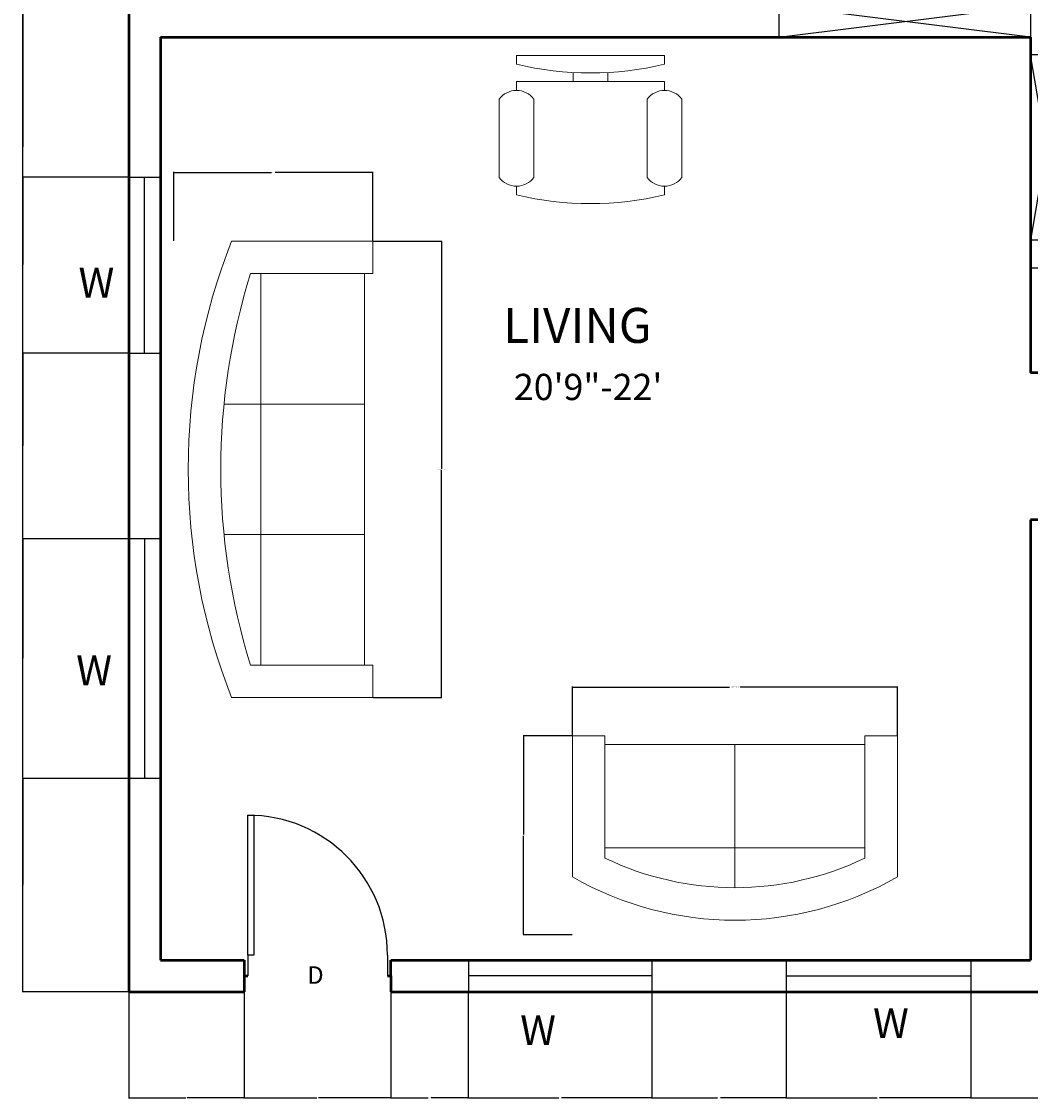
# Model space of a CAD drawing. Units: inches. Extents: x 2164 to 3752, y 2015 to 2629.
# Tile 5 of 8: x 3295 to 3583, y 2015 to 2323. Entities that reach past the tile are written whole.
import ezdxf
from ezdxf.enums import TextEntityAlignment as Align

# ---------------------------------------------------------------- set-up
doc = ezdxf.new("R2010")
doc.units = ezdxf.units.IN
for name, color, linetype, lineweight in [('A-ANNO-DIMS', 2, 'Continuous', 18), ('A-ANNO-TEXT', 7, 'Continuous', 25), ('A-AREA-IDEN', 3, 'Continuous', 25), ('A-DOOR', 3, 'Continuous', 25), ('A-FURN', 8, 'Continuous', 18), ('A-GLAZ', 4, 'Continuous', 25), ('A-WALL', 7, 'Continuous', 50)]:
    doc.layers.add(name, color=color, linetype=linetype, lineweight=lineweight)
doc.styles.get("Standard").update_dxf_attribs({"font": 'arial.ttf'})
doc.dimstyles.get("Standard").update_dxf_attribs({"dimtxt": 0.18, "dimasz": 0.18, "dimexe": 0.18, "dimexo": 0.0625, "dimgap": 0.09, "dimtad": 0, "dimtih": 1, "dimtoh": 1, "dimdec": 4, "dimzin": 0, "dimdsep": 46, "dimtxsty": 'Standard', "dimcen": 0.09, "dimadec": 0, "dimazin": 0, "dimtfac": 1, "dimtdec": 4, "dimtofl": 0, "dimtmove": 0, "dimatfit": 3, "dimfxl": 1, "dimtolj": 1, "dimtzin": 0, "dimarcsym": 0})

# ---------------------------------------------------------------- blocks, each defined once
blk = doc.blocks.new('*U7')
for p, q in [((0, 0), (0, -6)), ((40, 0), (40, -6))]:
    blk.add_line(p, q)
blk.add_lwpolyline([(0, 0), (0, 40), (1.75, 40), (1.75, 0)], close=True)
blk.add_arc((0, 0), 40, 0, 90)
blk = doc.blocks.new('Sofa - Roundback 7 ft.')
for p, q in [((-12.00002, -32.4421), (-12.00003, -6.5971)), ((11.99997, -32.4421), (11.99998, -6.5971)), ((-36.000027, -34), (-36.000027, -11.4696)), ((35.99998, -34), (35.99998, -11.4696)), ((-35.999844, -13.3819), (35.9998, -13.3819)), ((-36.000027, -32.4421), (35.99998, -32.4421))]:
    blk.add_line(p, q)
for points in [[(-36.000027, -34), (-42.000027, -34), (-42.000027, -8)], [(41.99998, -8), (41.99998, -34), (35.99998, -34)]]:
    blk.add_lwpolyline(points)
for centre, radius, start, end in [((0, -114.25), 114.25, 68.43141, 111.5686), ((-0.00001, -127.1968), 121.1968, 72.72033, 107.2797)]:
    blk.add_arc(centre, radius, start, end)
blk = doc.blocks.new('Sofa - Roundback Loveseat 5 ft.')
for p, q in [((0, -32.44198), (0, -5.99998)), ((-24, -33.99998), (-24, -11.46958)), ((24.00004, -33.99998), (24.00004, -11.46958)), ((-23.9998, -13.38178), (23.99986, -13.38178)), ((-24, -32.44198), (24.00004, -32.44198))]:
    blk.add_line(p, q)
for points in [[(-24, -33.99998), (-30, -33.99998), (-30, -7.99998)], [(30.00004, -7.99998), (30.00004, -33.99998), (24.00004, -33.99998)]]:
    blk.add_lwpolyline(points)
for centre, radius, start, end in [((0, -60.24998), 60.24998, 60.13715, 119.8628), ((0, -61.38438), 55.38444, 64.32083, 115.6792)]:
    blk.add_arc(centre, radius, start, end)
blk = doc.blocks.new('Chair - Desk')
for p, q in [((-8.5, 0), (-8.5, -1)), ((-8.5, 0), (8.5, 0)), ((8.5, 0), (8.5, -1)), ((-2, -3), (-2, -1.9355)), ((2, -1.9576), (2, -3)), ((-8.5, -3), (-8.5, -4)), ((-8.5, -3), (8.5, -3)), ((8.5, -3), (8.5, -4)), ((-10.5, -5), (-10.5, -14)), ((-6.5, -14), (-6.5, -5)), ((6.5, -5), (6.5, -14)), ((10.5, -14), (10.5, -5)), ((-8.5, -15), (-8.5, -16)), ((8.5, -15), (8.5, -16))]:
    blk.add_line(p, q)
for centre, radius, start, end in [((0, 34.625), 36.625, 256.5803, 283.4197), ((-8.5, -6.5), 2.5, 36.8699, 143.1301), ((8.5, -6.5), 2.5, 36.8699, 143.1301), ((-8.5, -12.5), 2.5, 216.8699, 323.1301), ((8.5, -12.5), 2.5, 216.8699, 323.1301), ((0, 19.625), 36.625, 256.5803, 283.4197)]:
    blk.add_arc(centre, radius, start, end)
blk = doc.blocks.new('VENT-OPENING')
for p, q in [((9, 53), (0, 53)), ((9, 53), (0, 0)), ((9, 0), (0, 53)), ((9, 0), (0, 0))]:
    blk.add_line(p, q)
blk = doc.blocks.new('*D27')
at = {"layer": 'A-ANNO-DIMS', "color": 0, "lineweight": -2, "transparency": 16777216}
for p, q in [((3395.28, 2260.44), (3414.99, 2260.44)), ((3414.81, 2260.26), (3414.81, 2195.32)), ((3414.81, 2130.01), (3414.81, 2194.95)), ((3395.28, 2129.83), (3414.99, 2129.83))]:
    blk.add_line(p, q, dxfattribs=at)
at = {"layer": 'A-ANNO-DIMS', "color": 0, "transparency": 16777216}
for points in [[(3414.78, 2260.26), (3414.84, 2260.26), (3414.81, 2260.44)], [(3414.78, 2130.01), (3414.84, 2130.01), (3414.81, 2129.83)]]:
    blk.add_solid(points, dxfattribs=at)
at = {"layer": 'Defpoints', "color": 0, "transparency": 16777216}
for p in [(3395.22, 2260.44), (3414.81, 2260.44), (3395.22, 2129.83)]:
    blk.add_point(p, dxfattribs=at)
at = {"layer": 'A-ANNO-DIMS', "color": 0, "transparency": 16777216, "insert": (3414.81, 2195.13), "char_height": 0.18, "attachment_point": 5}
blk.add_mtext('\\A1;SOFA 7 FT 131 TYP.', dxfattribs=at)
blk = doc.blocks.new('*D28')
at = {"layer": 'A-ANNO-DIMS', "color": 0, "lineweight": -2, "transparency": 16777216}
for p, q in [((3338.21, 2260.5), (3338.21, 2280.21)), ((3338.39, 2280.03), (3366.19, 2280.03)), ((3395.04, 2280.03), (3367.24, 2280.03)), ((3395.22, 2260.5), (3395.22, 2280.21))]:
    blk.add_line(p, q, dxfattribs=at)
at = {"layer": 'A-ANNO-DIMS', "color": 0, "transparency": 16777216}
for points in [[(3338.39, 2280.06), (3338.39, 2280), (3338.21, 2280.03)], [(3395.04, 2280.06), (3395.04, 2280), (3395.22, 2280.03)]]:
    blk.add_solid(points, dxfattribs=at)
at = {"layer": 'Defpoints', "color": 0, "transparency": 16777216}
for p in [(3338.21, 2280.03), (3338.21, 2260.44), (3395.22, 2260.44)]:
    blk.add_point(p, dxfattribs=at)
at = {"layer": 'A-ANNO-DIMS', "color": 0, "transparency": 16777216, "insert": (3366.72, 2280.03), "char_height": 0.18, "attachment_point": 5}
blk.add_mtext('\\A1;57 TYP.', dxfattribs=at)
blk = doc.blocks.new('*D29')
at = {"layer": 'A-ANNO-DIMS', "color": 0, "lineweight": -2, "transparency": 16777216}
for p, q in [((3452.32, 2118.94), (3452.32, 2133.02)), ((3452.5, 2132.84), (3497.31, 2132.84)), ((3545.16, 2132.84), (3500.34, 2132.84)), ((3545.34, 2118.94), (3545.34, 2133.02))]:
    blk.add_line(p, q, dxfattribs=at)
at = {"layer": 'A-ANNO-DIMS', "color": 0, "transparency": 16777216}
for points in [[(3452.5, 2132.87), (3452.5, 2132.81), (3452.32, 2132.84)], [(3545.16, 2132.87), (3545.16, 2132.81), (3545.34, 2132.84)]]:
    blk.add_solid(points, dxfattribs=at)
at = {"layer": 'Defpoints', "color": 0, "transparency": 16777216}
for p in [(3452.32, 2132.84), (3452.32, 2118.88), (3545.34, 2118.88)]:
    blk.add_point(p, dxfattribs=at)
at = {"layer": 'A-ANNO-DIMS', "color": 0, "transparency": 16777216, "insert": (3498.83, 2132.84), "char_height": 0.18, "attachment_point": 5}
blk.add_mtext('\\A1;LOVESEAT 5 FT 93 TYP.', dxfattribs=at)
blk = doc.blocks.new('*D30')
at = {"layer": 'A-ANNO-DIMS', "color": 0, "lineweight": -2, "transparency": 16777216}
for p, q in [((3452.25, 2118.88), (3438.18, 2118.88)), ((3438.36, 2118.7), (3438.36, 2090.64)), ((3438.36, 2062.21), (3438.36, 2090.28)), ((3452.25, 2062.03), (3438.18, 2062.03))]:
    blk.add_line(p, q, dxfattribs=at)
at = {"layer": 'A-ANNO-DIMS', "color": 0, "transparency": 16777216}
for points in [[(3438.33, 2118.7), (3438.39, 2118.7), (3438.36, 2118.88)], [(3438.33, 2062.21), (3438.39, 2062.21), (3438.36, 2062.03)]]:
    blk.add_solid(points, dxfattribs=at)
at = {"layer": 'Defpoints', "color": 0, "transparency": 16777216}
for p in [(3452.32, 2118.88), (3438.36, 2062.03), (3452.32, 2062.03)]:
    blk.add_point(p, dxfattribs=at)
at = {"layer": 'A-ANNO-DIMS', "color": 0, "transparency": 16777216, "insert": (3438.36, 2090.46), "char_height": 0.18, "attachment_point": 5}
blk.add_mtext('\\A1;57 TYP.', dxfattribs=at)
blk = doc.blocks.new('*D34')
at = {"layer": 'A-ANNO-DIMS', "color": 0, "lineweight": -2, "transparency": 16777216}
for p, q in [((3583.39, 2260.65), (3583.39, 2252.59)), ((3592.39, 2260.65), (3592.39, 2252.59)), ((3583.57, 2252.77), (3587.44, 2252.77)), ((3592.21, 2252.77), (3588.35, 2252.77))]:
    blk.add_line(p, q, dxfattribs=at)
at = {"layer": 'A-ANNO-DIMS', "color": 0, "transparency": 16777216}
for points in [[(3583.57, 2252.8), (3583.57, 2252.74), (3583.39, 2252.77)], [(3592.21, 2252.8), (3592.21, 2252.74), (3592.39, 2252.77)]]:
    blk.add_solid(points, dxfattribs=at)
at = {"layer": 'Defpoints', "color": 0, "transparency": 16777216}
for p in [(3583.39, 2260.72), (3592.39, 2260.72), (3592.39, 2252.77)]:
    blk.add_point(p, dxfattribs=at)
at = {"layer": 'A-ANNO-DIMS', "color": 0, "transparency": 16777216, "insert": (3587.89, 2252.77), "char_height": 0.18, "attachment_point": 5}
blk.add_mtext('\\A1;9 TYP.', dxfattribs=at)
blk = doc.blocks.new('*D111')
at = {"layer": 'A-ANNO-DIMS', "color": 0, "lineweight": -2, "transparency": 16777216}
for p, q in [((3325.39, 2045.65), (3325.39, 2015.19)), ((3358.39, 2045.65), (3358.39, 2015.19)), ((3325.57, 2015.37), (3341.68, 2015.37)), ((3358.21, 2015.37), (3342.11, 2015.37))]:
    blk.add_line(p, q, dxfattribs=at)
at = {"layer": 'A-ANNO-DIMS', "color": 0, "transparency": 16777216}
for points in [[(3325.57, 2015.4), (3325.57, 2015.34), (3325.39, 2015.37)], [(3358.21, 2015.4), (3358.21, 2015.34), (3358.39, 2015.37)]]:
    blk.add_solid(points, dxfattribs=at)
at = {"layer": 'Defpoints', "color": 0, "transparency": 16777216}
for p in [(3325.39, 2045.72), (3358.39, 2045.72), (3358.39, 2015.37)]:
    blk.add_point(p, dxfattribs=at)
at = {"layer": 'A-ANNO-DIMS', "color": 0, "transparency": 16777216, "insert": (3341.89, 2015.37), "char_height": 0.18, "attachment_point": 5}
blk.add_mtext('\\A1;33', dxfattribs=at)
blk = doc.blocks.new('*D112')
at = {"layer": 'A-ANNO-DIMS', "color": 0, "lineweight": -2, "transparency": 16777216}
for p, q in [((3358.39, 2045.65), (3358.39, 2015.19)), ((3400.39, 2045.65), (3400.39, 2015.19)), ((3358.57, 2015.37), (3379.17, 2015.37)), ((3400.21, 2015.37), (3379.62, 2015.37))]:
    blk.add_line(p, q, dxfattribs=at)
at = {"layer": 'A-ANNO-DIMS', "color": 0, "transparency": 16777216}
for points in [[(3358.57, 2015.4), (3358.57, 2015.34), (3358.39, 2015.37)], [(3400.21, 2015.4), (3400.21, 2015.34), (3400.39, 2015.37)]]:
    blk.add_solid(points, dxfattribs=at)
at = {"layer": 'Defpoints', "color": 0, "transparency": 16777216}
for p in [(3358.39, 2045.72), (3400.39, 2045.72), (3400.39, 2015.37)]:
    blk.add_point(p, dxfattribs=at)
at = {"layer": 'A-ANNO-DIMS', "color": 0, "transparency": 16777216, "insert": (3379.39, 2015.37), "char_height": 0.18, "attachment_point": 5}
blk.add_mtext('\\A1;42', dxfattribs=at)
blk = doc.blocks.new('*D113')
at = {"layer": 'A-ANNO-DIMS', "color": 0, "lineweight": -2, "transparency": 16777216}
for p, q in [((3400.39, 2045.65), (3400.39, 2015.19)), ((3422.53, 2045.65), (3422.53, 2015.19)), ((3400.57, 2015.37), (3411, 2015.37)), ((3422.35, 2015.37), (3411.93, 2015.37))]:
    blk.add_line(p, q, dxfattribs=at)
at = {"layer": 'A-ANNO-DIMS', "color": 0, "transparency": 16777216}
for points in [[(3400.57, 2015.4), (3400.57, 2015.34), (3400.39, 2015.37)], [(3422.35, 2015.4), (3422.35, 2015.34), (3422.53, 2015.37)]]:
    blk.add_solid(points, dxfattribs=at)
at = {"layer": 'Defpoints', "color": 0, "transparency": 16777216}
for p in [(3400.39, 2045.72), (3422.53, 2045.72), (3422.53, 2015.37)]:
    blk.add_point(p, dxfattribs=at)
at = {"layer": 'A-ANNO-DIMS', "color": 0, "transparency": 16777216, "insert": (3411.46, 2015.37), "char_height": 0.18, "attachment_point": 5}
blk.add_mtext('\\A1;22.137', dxfattribs=at)
blk = doc.blocks.new('*D114')
at = {"layer": 'A-ANNO-DIMS', "color": 0, "lineweight": -2, "transparency": 16777216}
for p, q in [((3422.53, 2045.65), (3422.53, 2015.19)), ((3475.06, 2045.65), (3475.06, 2015.19)), ((3422.71, 2015.37), (3448.4, 2015.37)), ((3474.88, 2015.37), (3449.19, 2015.37))]:
    blk.add_line(p, q, dxfattribs=at)
at = {"layer": 'A-ANNO-DIMS', "color": 0, "transparency": 16777216}
for points in [[(3422.71, 2015.4), (3422.71, 2015.34), (3422.53, 2015.37)], [(3474.88, 2015.4), (3474.88, 2015.34), (3475.06, 2015.37)]]:
    blk.add_solid(points, dxfattribs=at)
at = {"layer": 'Defpoints', "color": 0, "transparency": 16777216}
for p in [(3422.53, 2045.72), (3475.06, 2045.72), (3475.06, 2015.37)]:
    blk.add_point(p, dxfattribs=at)
at = {"layer": 'A-ANNO-DIMS', "color": 0, "transparency": 16777216, "insert": (3448.8, 2015.37), "char_height": 0.18, "attachment_point": 5}
blk.add_mtext('\\A1;52.53', dxfattribs=at)
blk = doc.blocks.new('*D115')
at = {"layer": 'A-ANNO-DIMS', "color": 0, "lineweight": -2, "transparency": 16777216}
for p, q in [((3475.06, 2045.65), (3475.06, 2015.19)), ((3513.44, 2045.65), (3513.44, 2015.19)), ((3475.24, 2015.37), (3493.79, 2015.37)), ((3513.26, 2015.37), (3494.71, 2015.37))]:
    blk.add_line(p, q, dxfattribs=at)
at = {"layer": 'A-ANNO-DIMS', "color": 0, "transparency": 16777216}
for points in [[(3475.24, 2015.4), (3475.24, 2015.34), (3475.06, 2015.37)], [(3513.26, 2015.4), (3513.26, 2015.34), (3513.44, 2015.37)]]:
    blk.add_solid(points, dxfattribs=at)
at = {"layer": 'Defpoints', "color": 0, "transparency": 16777216}
for p in [(3475.06, 2045.72), (3513.44, 2045.72), (3513.44, 2015.37)]:
    blk.add_point(p, dxfattribs=at)
at = {"layer": 'A-ANNO-DIMS', "color": 0, "transparency": 16777216, "insert": (3494.25, 2015.37), "char_height": 0.18, "attachment_point": 5}
blk.add_mtext('\\A1;38.374', dxfattribs=at)
blk = doc.blocks.new('*D116')
at = {"layer": 'A-ANNO-DIMS', "color": 0, "lineweight": -2, "transparency": 16777216}
for p, q in [((3513.44, 2045.65), (3513.44, 2015.19)), ((3566.34, 2045.65), (3566.34, 2015.19)), ((3513.62, 2015.37), (3539.57, 2015.37)), ((3566.16, 2015.37), (3540.21, 2015.37))]:
    blk.add_line(p, q, dxfattribs=at)
at = {"layer": 'A-ANNO-DIMS', "color": 0, "transparency": 16777216}
for points in [[(3513.62, 2015.4), (3513.62, 2015.34), (3513.44, 2015.37)], [(3566.16, 2015.4), (3566.16, 2015.34), (3566.34, 2015.37)]]:
    blk.add_solid(points, dxfattribs=at)
at = {"layer": 'Defpoints', "color": 0, "transparency": 16777216}
for p in [(3513.44, 2045.72), (3566.34, 2045.72), (3566.34, 2015.37)]:
    blk.add_point(p, dxfattribs=at)
at = {"layer": 'A-ANNO-DIMS', "color": 0, "transparency": 16777216, "insert": (3539.89, 2015.37), "char_height": 0.18, "attachment_point": 5}
blk.add_mtext('\\A1;52.9', dxfattribs=at)
blk = doc.blocks.new('*D117')
at = {"layer": 'A-ANNO-DIMS', "color": 0, "lineweight": -2, "transparency": 16777216}
for p, q in [((3566.34, 2045.65), (3566.34, 2015.19)), ((3626.11, 2045.65), (3626.11, 2015.19)), ((3566.52, 2015.37), (3595.83, 2015.37)), ((3625.93, 2015.37), (3596.62, 2015.37))]:
    blk.add_line(p, q, dxfattribs=at)
at = {"layer": 'A-ANNO-DIMS', "color": 0, "transparency": 16777216}
for points in [[(3566.52, 2015.4), (3566.52, 2015.34), (3566.34, 2015.37)], [(3625.93, 2015.4), (3625.93, 2015.34), (3626.11, 2015.37)]]:
    blk.add_solid(points, dxfattribs=at)
at = {"layer": 'Defpoints', "color": 0, "transparency": 16777216}
for p in [(3566.34, 2045.72), (3626.11, 2045.72), (3626.11, 2015.37)]:
    blk.add_point(p, dxfattribs=at)
at = {"layer": 'A-ANNO-DIMS', "color": 0, "transparency": 16777216, "insert": (3596.23, 2015.37), "char_height": 0.18, "attachment_point": 5}
blk.add_mtext('\\A1;59.77', dxfattribs=at)
blk = doc.blocks.new('*D120')
at = {"layer": 'A-ANNO-DIMS', "color": 0, "lineweight": -2, "transparency": 16777216}
for p, q in [((3325.33, 2106.67), (3294.86, 2106.67)), ((3295.04, 2106.49), (3295.04, 2076.37)), ((3295.04, 2045.9), (3295.04, 2076.01)), ((3325.33, 2045.72), (3294.86, 2045.72))]:
    blk.add_line(p, q, dxfattribs=at)
at = {"layer": 'A-ANNO-DIMS', "color": 0, "transparency": 16777216}
for points in [[(3295.01, 2106.49), (3295.07, 2106.49), (3295.04, 2106.67)], [(3295.01, 2045.9), (3295.07, 2045.9), (3295.04, 2045.72)]]:
    blk.add_solid(points, dxfattribs=at)
at = {"layer": 'Defpoints', "color": 0, "transparency": 16777216}
for p in [(3295.04, 2106.67), (3325.39, 2106.67), (3325.39, 2045.72)]:
    blk.add_point(p, dxfattribs=at)
at = {"layer": 'A-ANNO-DIMS', "color": 0, "transparency": 16777216, "insert": (3295.04, 2076.19), "char_height": 0.18, "attachment_point": 5}
blk.add_mtext('\\A1;60.95', dxfattribs=at)
blk = doc.blocks.new('*D121')
at = {"layer": 'A-ANNO-DIMS', "color": 0, "lineweight": -2, "transparency": 16777216}
for p, q in [((3325.33, 2175.28), (3294.86, 2175.28)), ((3295.04, 2175.1), (3295.04, 2141.16)), ((3295.04, 2106.85), (3295.04, 2140.79)), ((3325.33, 2106.67), (3294.86, 2106.67))]:
    blk.add_line(p, q, dxfattribs=at)
at = {"layer": 'A-ANNO-DIMS', "color": 0, "transparency": 16777216}
for points in [[(3295.01, 2175.1), (3295.07, 2175.1), (3295.04, 2175.28)], [(3295.01, 2106.85), (3295.07, 2106.85), (3295.04, 2106.67)]]:
    blk.add_solid(points, dxfattribs=at)
at = {"layer": 'Defpoints', "color": 0, "transparency": 16777216}
for p in [(3295.04, 2175.28), (3325.39, 2175.28), (3325.39, 2106.67)]:
    blk.add_point(p, dxfattribs=at)
at = {"layer": 'A-ANNO-DIMS', "color": 0, "transparency": 16777216, "insert": (3295.04, 2140.97), "char_height": 0.18, "attachment_point": 5}
blk.add_mtext('\\A1;68.61', dxfattribs=at)
blk = doc.blocks.new('*D122')
at = {"layer": 'A-ANNO-DIMS', "color": 0, "lineweight": -2, "transparency": 16777216}
for p, q in [((3325.33, 2228.35), (3294.86, 2228.35)), ((3295.04, 2228.17), (3295.04, 2202)), ((3295.04, 2175.46), (3295.04, 2201.63)), ((3325.33, 2175.28), (3294.86, 2175.28))]:
    blk.add_line(p, q, dxfattribs=at)
at = {"layer": 'A-ANNO-DIMS', "color": 0, "transparency": 16777216}
for points in [[(3295.01, 2228.17), (3295.07, 2228.17), (3295.04, 2228.35)], [(3295.01, 2175.46), (3295.07, 2175.46), (3295.04, 2175.28)]]:
    blk.add_solid(points, dxfattribs=at)
at = {"layer": 'Defpoints', "color": 0, "transparency": 16777216}
for p in [(3295.04, 2228.35), (3325.39, 2228.35), (3325.39, 2175.28)]:
    blk.add_point(p, dxfattribs=at)
at = {"layer": 'A-ANNO-DIMS', "color": 0, "transparency": 16777216, "insert": (3295.04, 2201.82), "char_height": 0.18, "attachment_point": 5}
blk.add_mtext('\\A1;53.07', dxfattribs=at)
blk = doc.blocks.new('*D123')
at = {"layer": 'A-ANNO-DIMS', "color": 0, "lineweight": -2, "transparency": 16777216}
for p, q in [((3325.33, 2278.69), (3294.86, 2278.69)), ((3295.04, 2278.51), (3295.04, 2253.7)), ((3295.04, 2228.53), (3295.04, 2253.34)), ((3325.33, 2228.35), (3294.86, 2228.35))]:
    blk.add_line(p, q, dxfattribs=at)
at = {"layer": 'A-ANNO-DIMS', "color": 0, "transparency": 16777216}
for points in [[(3295.01, 2278.51), (3295.07, 2278.51), (3295.04, 2278.69)], [(3295.01, 2228.53), (3295.07, 2228.53), (3295.04, 2228.35)]]:
    blk.add_solid(points, dxfattribs=at)
at = {"layer": 'Defpoints', "color": 0, "transparency": 16777216}
for p in [(3295.04, 2278.69), (3325.39, 2278.69), (3325.39, 2228.35)]:
    blk.add_point(p, dxfattribs=at)
at = {"layer": 'A-ANNO-DIMS', "color": 0, "transparency": 16777216, "insert": (3295.04, 2253.52), "char_height": 0.18, "attachment_point": 5}
blk.add_mtext('\\A1;50.34', dxfattribs=at)
blk = doc.blocks.new('*D124')
at = {"layer": 'A-ANNO-DIMS', "color": 0, "lineweight": -2, "transparency": 16777216}
for p, q in [((3325.33, 2395.15), (3294.86, 2395.15)), ((3295.04, 2394.97), (3295.04, 2337.1)), ((3295.04, 2278.87), (3295.04, 2336.74)), ((3325.33, 2278.69), (3294.86, 2278.69))]:
    blk.add_line(p, q, dxfattribs=at)
at = {"layer": 'A-ANNO-DIMS', "color": 0, "transparency": 16777216}
for points in [[(3295.01, 2394.97), (3295.07, 2394.97), (3295.04, 2395.15)], [(3295.01, 2278.87), (3295.07, 2278.87), (3295.04, 2278.69)]]:
    blk.add_solid(points, dxfattribs=at)
at = {"layer": 'Defpoints', "color": 0, "transparency": 16777216}
for p in [(3295.04, 2395.15), (3325.39, 2395.15), (3325.39, 2278.69)]:
    blk.add_point(p, dxfattribs=at)
at = {"layer": 'A-ANNO-DIMS', "color": 0, "transparency": 16777216, "insert": (3295.04, 2336.92), "char_height": 0.18, "attachment_point": 5}
blk.add_mtext('\\A1;116.47', dxfattribs=at)
blk = doc.blocks.new('*D127')
at = {"layer": 'A-ANNO-DIMS', "color": 0, "lineweight": -2, "transparency": 16777216}
for p, q in [((3325.33, 2528.72), (3294.86, 2528.72)), ((3295.04, 2528.54), (3295.04, 2287.4)), ((3295.04, 2045.9), (3295.04, 2287.04)), ((3325.33, 2045.72), (3294.86, 2045.72))]:
    blk.add_line(p, q, dxfattribs=at)
at = {"layer": 'A-ANNO-DIMS', "color": 0, "transparency": 16777216}
for points in [[(3295.01, 2528.54), (3295.07, 2528.54), (3295.04, 2528.72)], [(3295.01, 2045.9), (3295.07, 2045.9), (3295.04, 2045.72)]]:
    blk.add_solid(points, dxfattribs=at)
at = {"layer": 'Defpoints', "color": 0, "transparency": 16777216}
for p in [(3295.04, 2528.72), (3325.39, 2528.72), (3325.39, 2045.72)]:
    blk.add_point(p, dxfattribs=at)
at = {"layer": 'A-ANNO-DIMS', "color": 0, "transparency": 16777216, "insert": (3295.04, 2287.22), "char_height": 0.18, "attachment_point": 5}
blk.add_mtext('\\A1;483', dxfattribs=at)

msp = doc.modelspace()

# ---------------------------------------------------------------- linework, layer by layer
at = {"layer": 'A-GLAZ'}
for p, q in [((3511.395, 2327.7172), (3511.395, 2318.7172)), ((3511.395, 2318.7172), (3583.395, 2327.7172)), ((3583.395, 2318.7172), (3511.395, 2327.7172)), ((3583.395, 2327.7172), (3583.395, 2318.7172)), ((3325.395, 2278.6856), (3334.395, 2278.6856)), ((3329.895, 2228.3505), (3329.895, 2278.6856)), ((3325.395, 2228.3505), (3334.395, 2228.3505)), ((3334.395, 2175.28), (3325.395, 2175.28)), ((3329.895, 2175.28), (3329.895, 2106.6668)), ((3334.395, 2106.6668), (3325.395, 2106.6668)), ((3422.5315, 2054.7172), (3422.5315, 2045.7172)), ((3475.0634, 2054.7172), (3475.0634, 2045.7172)), ((3513.4377, 2054.7172), (3513.4377, 2045.7172)), ((3566.3421, 2054.7172), (3566.3421, 2045.7172)), ((3475.0634, 2050.2172), (3422.5315, 2050.2172)), ((3513.4377, 2050.2172), (3566.3421, 2050.2172))]:
    msp.add_line(p, q, dxfattribs=at)
at = {"layer": 'A-WALL'}
for p, q in [((3325.395, 2528.7172), (3325.395, 2045.7172)), ((3334.395, 2318.7172), (3583.395, 2318.7172)), ((3334.395, 2318.7172), (3334.395, 2054.7172)), ((3511.395, 2318.7172), (3583.395, 2318.7172)), ((3583.395, 2318.7172), (3583.395, 2222.7172)), ((3592.395, 2222.7172), (3583.395, 2222.7172)), ((3587.895, 2180.7172), (3583.395, 2180.7172)), ((3583.395, 2180.7172), (3583.395, 2054.7172)), ((3334.395, 2054.7172), (3358.395, 2054.7172)), ((3358.395, 2054.7172), (3358.395, 2045.7172)), ((3400.395, 2050.2172), (3400.395, 2054.7172)), ((3400.395, 2054.7172), (3583.395, 2054.7172)), ((3511.395, 2054.7172), (3583.395, 2054.7172)), ((3358.395, 2050.2172), (3359.395, 2050.2172)), ((3399.395, 2050.2172), (3400.395, 2050.2172)), ((3400.395, 2050.2172), (3400.395, 2045.7172)), ((3325.395, 2045.7172), (3358.395, 2045.7172)), ((3400.395, 2045.7172), (3721.395, 2045.7172))]:
    msp.add_line(p, q, dxfattribs=at)

# ---------------------------------------------------------------- block references
at = {"layer": 'A-DOOR'}
msp.add_blockref('*U7', (3359.395, 2056.2172), dxfattribs=at)
at = {"layer": 'A-FURN', "xscale": 2.491772613573976, "yscale": 2.491772613573976, "zscale": 2.491772613573976}
msp.add_blockref('Chair - Desk', (3457.4842, 2313.4971), dxfattribs=at)
at = {"layer": 'A-FURN'}
for name, p, xscale, yscale, zscale, rotation in [('Sofa - Roundback 7 ft.', (3342.356, 2195.1336), 1.554837866346122, 1.554837866346122, 1.554837866346122, 90), ('Sofa - Roundback Loveseat 5 ft.', (3498.8272, 2066.1683), 1.550400962032466, 1.550400962032466, 1.550400962032466, 180)]:
    msp.add_blockref(name, p, dxfattribs=dict(at, xscale=xscale, yscale=yscale, zscale=zscale, rotation=rotation))
at = {"layer": 'A-GLAZ'}
msp.add_blockref('VENT-OPENING', (3583.395, 2260.717), dxfattribs=at)

# ---------------------------------------------------------------- texts
at = {"layer": 'A-ANNO-TEXT'}
for p in [(3316.1032, 2247.4164), (3315.4345, 2136.5052), (3543.4583, 2035.616), (3442.4859, 2033.6116)]:
    msp.add_text('W', height=8.5558, dxfattribs=at).set_placement(p, align=Align.MIDDLE)
msp.add_text('D', height=5, dxfattribs=at).set_placement((3376.4343, 2047.9828))
at = {"layer": 'A-AREA-IDEN'}
for s, height, p in [('LIVING', 10, (3432.4885, 2231.305)), ('20\'9"-22\'', 7.5, (3435.5698, 2214.9483))]:
    msp.add_text(s, height=height, dxfattribs=at).set_placement(p)

# ---------------------------------------------------------------- dimensions: what is measured, and where the dimension line sits
at = {"layer": 'A-ANNO-DIMS'}
for base, p1, p2, override, picture, middle in [((3295.045, 2528.7172), (3325.395, 2045.7172), (3325.395, 2528.7172), {"dimdec": 0, "dimlfac": 1, "dimrnd": 0, "dimzin": 0, "dimdsep": 46, "dimlunit": 2}, '*D127', (3295.045, 2287.2172)), ((3295.045, 2395.1516), (3325.395, 2278.6856), (3325.395, 2395.1516), {"dimdec": 2, "dimlfac": 1, "dimrnd": 0, "dimzin": 0, "dimdsep": 46, "dimlunit": 2}, '*D124', (3295.045, 2336.9186)), ((3295.045, 2278.6856), (3325.395, 2228.3505), (3325.395, 2278.6856), {"dimdec": 2, "dimlfac": 1, "dimrnd": 0, "dimzin": 0, "dimdsep": 46, "dimlunit": 2}, '*D123', (3295.045, 2253.5181)), ((3295.045, 2228.3505), (3325.395, 2175.28), (3325.395, 2228.3505), {"dimdec": 2, "dimlfac": 1, "dimrnd": 0, "dimzin": 0, "dimdsep": 46, "dimlunit": 2}, '*D122', (3295.045, 2201.8152)), ((3295.045, 2175.28), (3325.395, 2106.6668), (3325.395, 2175.28), {"dimdec": 2, "dimlfac": 1, "dimrnd": 0, "dimzin": 0, "dimdsep": 46, "dimlunit": 2}, '*D121', (3295.045, 2140.9734)), ((3295.045, 2106.6668), (3325.395, 2045.7172), (3325.395, 2106.6668), {"dimdec": 2, "dimlfac": 1, "dimrnd": 0, "dimzin": 0, "dimdsep": 46, "dimlunit": 2}, '*D120', (3295.045, 2076.192))]:
    dim = msp.add_linear_dim(base=base, p1=p1, p2=p2, angle=90, dimstyle='Standard', override=override, dxfattribs=at)
    dim.commit()
    dim.dimension.update_dxf_attribs({"geometry": picture, "text_midpoint": middle})
for base, p1, p2, angle, text, picture, middle in [((3338.2097, 2280.0278), (3395.2205, 2260.4368), (3338.2097, 2260.4368), 180, '<> TYP.', '*D28', (3366.7151, 2280.0278)), ((3414.8114, 2260.4368), (3395.2205, 2129.8304), (3395.2205, 2260.4368), 90, 'SOFA 7 FT <> TYP.', '*D27', (3414.8114, 2195.1336)), ((3452.3151, 2132.8355), (3545.3392, 2118.8819), (3452.3151, 2118.8819), 180, 'LOVESEAT 5 FT <> TYP.', '*D29', (3498.8271, 2132.8355)), ((3438.3614, 2062.0339), (3452.3151, 2118.8819), (3452.3151, 2062.0339), 270, '<> TYP.', '*D30', (3438.3614, 2090.4579))]:
    dim = msp.add_linear_dim(base=base, p1=p1, p2=p2, angle=angle, text=text, dimstyle='Standard', override={"dimdec": 0, "dimrnd": 0, "dimzin": 0, "dimlunit": 2}, dxfattribs=at)
    dim.commit()
    dim.dimension.update_dxf_attribs({"geometry": picture, "text_midpoint": middle})
dim = msp.add_linear_dim(base=(3592.395, 2252.7672), p1=(3583.395, 2260.7172), p2=(3592.395, 2260.7172), text='<> TYP.', dimstyle='Standard', override={"dimdec": 0, "dimrnd": 0, "dimzin": 0, "dimlunit": 2}, dxfattribs=at)
dim.commit()
dim.dimension.update_dxf_attribs({"geometry": '*D34', "text_midpoint": (3587.895, 2252.7672)})
for base, p1, p2, override, picture, middle in [((3358.395, 2015.3672), (3325.395, 2045.7172), (3358.395, 2045.7172), {"dimdec": 0, "dimlfac": 1, "dimrnd": 0, "dimzin": 0, "dimdsep": 46, "dimlunit": 2}, '*D111', (3341.895, 2015.3672)), ((3400.395, 2015.3672), (3358.395, 2045.7172), (3400.395, 2045.7172), {"dimdec": 0, "dimlfac": 1, "dimrnd": 0, "dimzin": 0, "dimdsep": 46, "dimlunit": 2}, '*D112', (3379.395, 2015.3672)), ((3422.53153, 2015.36725), (3400.39496, 2045.71725), (3422.53153, 2045.71725), {"dimdec": 3, "dimlfac": 1, "dimrnd": 0, "dimzin": 0, "dimdsep": 46, "dimlunit": 2}, '*D113', (3411.46325, 2015.36725)), ((3475.0634, 2015.3672), (3422.5315, 2045.7172), (3475.0634, 2045.7172), {"dimdec": 2, "dimlfac": 1, "dimrnd": 0, "dimzin": 0, "dimdsep": 46, "dimlunit": 2}, '*D114', (3448.7974, 2015.3672)), ((3513.4377, 2015.3672), (3475.0634, 2045.7172), (3513.4377, 2045.7172), {"dimdec": 3, "dimlfac": 1, "dimrnd": 0, "dimzin": 0, "dimdsep": 46, "dimlunit": 2}, '*D115', (3494.2505, 2015.3672)), ((3566.3421, 2015.3672), (3513.4377, 2045.7172), (3566.3421, 2045.7172), {"dimdec": 1, "dimlfac": 1, "dimrnd": 0, "dimzin": 0, "dimdsep": 46, "dimlunit": 2}, '*D116', (3539.8899, 2015.3672)), ((3626.1138, 2015.3672), (3566.3421, 2045.7172), (3626.1138, 2045.7172), {"dimdec": 2, "dimlfac": 1, "dimrnd": 0, "dimzin": 0, "dimdsep": 46, "dimlunit": 2}, '*D117', (3596.2279, 2015.3672))]:
    dim = msp.add_linear_dim(base=base, p1=p1, p2=p2, dimstyle='Standard', override=override, dxfattribs=at)
    dim.commit()
    dim.dimension.update_dxf_attribs({"geometry": picture, "text_midpoint": middle})

doc.saveas('drawing.dxf')
